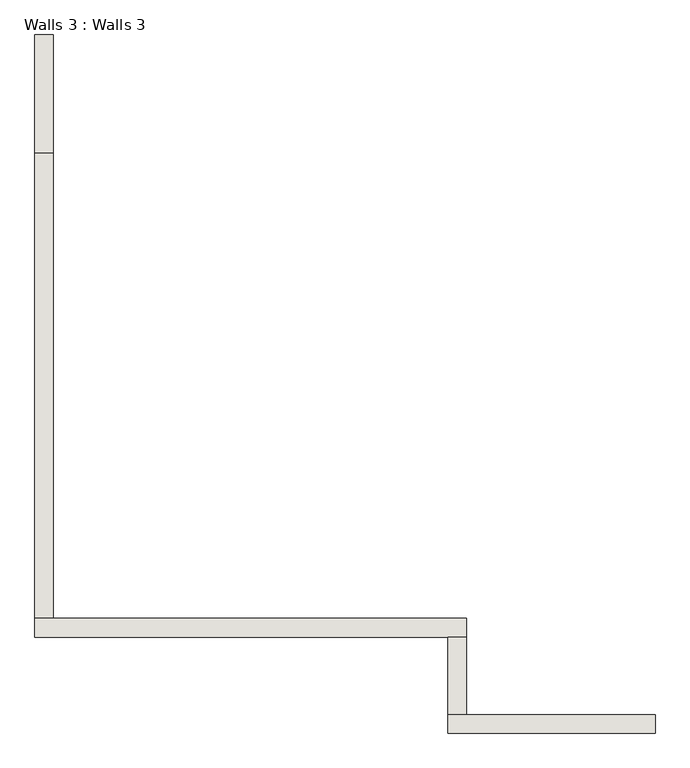
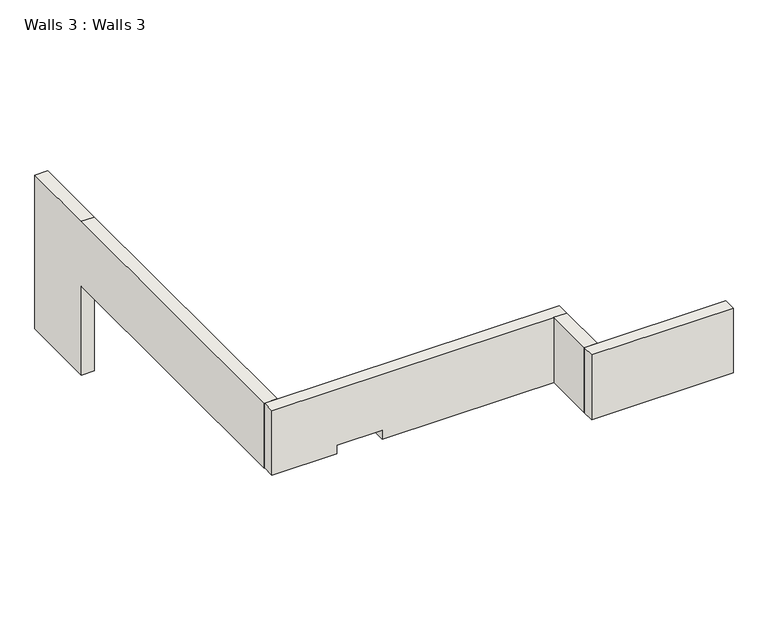
"""IFC4 building model written with IfcOpenShell, lengths in millimetres: wall geometry, Walls 3 : Walls 3."""

from ifc_helpers import new_model, si_unit, frame, origin, place, context, project, spatial, polyline, outline, extrude, source, transform, mapped, element, save


def walls_3_walls_3_ce3253ed(model_context):
    return source(origin(), model_context, "Body", "SweptSolid", [
        extrude(outline(polyline([(3726.6918749, -301.9046951), (-248.3207252, -301.9046951), (-248.3207252, 53.6953049), (3726.6918749, 53.6953049), (3726.6918749, -301.9046951)])), frame((0.0, 0.0, 8432.8), z_axis=(0.0, 0.0, 1.0), x_axis=(1.0, 0.0, 0.0)), (0.0, 0.0, 1.0), 1930.4),
        extrude(outline(polyline([(-248.3207252, 53.6953049), (-248.3207252, 1539.5953049), (107.2792748, 1539.5953049), (107.2792748, 53.6953049), (-248.3207252, 53.6953049)])), frame((0.0, 0.0, 8432.8), z_axis=(0.0, 0.0, 1.0), x_axis=(1.0, 0.0, 0.0)), (0.0, 0.0, 1.0), 1930.4),
        extrude(outline(polyline([(10363.2, 107.1918749), (10363.2, -8173.2081251), (8445.5, -8173.2081251), (8445.5, -6346.8069291), (8699.5, -6346.8069291), (8699.5, -5076.8069291), (8432.8, -5076.8069291), (8432.8, 107.1918749), (10363.2, 107.1918749)])), frame((0.0, 1539.5953049, 0.0), z_axis=(0.0, 1.0, 0.0), x_axis=(0.0, 0.0, 1.0)), (0.0, 0.0, 1.0), 355.6),
        extrude(outline(polyline([(10816.5055105, 5791.2), (10816.5055105, 8432.8), (1907.6881753, 8432.8), (1907.6881753, 10363.2), (10816.5055105, 10363.2), (13083.8953049, 10363.2), (13083.8953049, 5791.2), (10816.5055105, 5791.2)])), frame((-8173.2081251, 0.0, 0.0), z_axis=(1.0, 0.0, 0.0), x_axis=(0.0, 1.0, 0.0)), (0.0, 0.0, 1.0), 355.6),
    ])


if __name__ == "__main__":
    model = new_model("IFC4")
    model_context = context("Model", 3, world=origin())
    ifc_project = project(units=[si_unit("LENGTHUNIT", "METRE", prefix="MILLI")], contexts=[model_context])
    site = spatial("IfcSite", under=ifc_project)
    building = spatial("IfcBuilding", under=site)
    placement = place(None, origin())
    walls_3_walls_3_shape = walls_3_walls_3_ce3253ed(model_context)
    element("IfcWall", 1, ObjectType="Walls 3 : Walls 3", at=placement, inside=building, context=model_context, shape_type="MappedRepresentation", body=[
        mapped(walls_3_walls_3_shape, transform((0.0, 0.0, 0.0), x_axis=(1.0, 0.0, 0.0), y_axis=(0.0, 1.0, 0.0), z_axis=(0.0, 0.0, 1.0))),
    ])
    save(model, "model.ifc")

# Revit data of these elements
# Element 1 (IfcWall, "Walls 3 : Walls 3")
#   Materials on its faces: "1 white", "Default Wall"
# Materials
#   "1 white": class "Generic", colour RGB 244 245 241, transparency 0, Cost = 0
#   "Default Wall": colour RGB 128 128 128, transparency 0, Cost = 0
